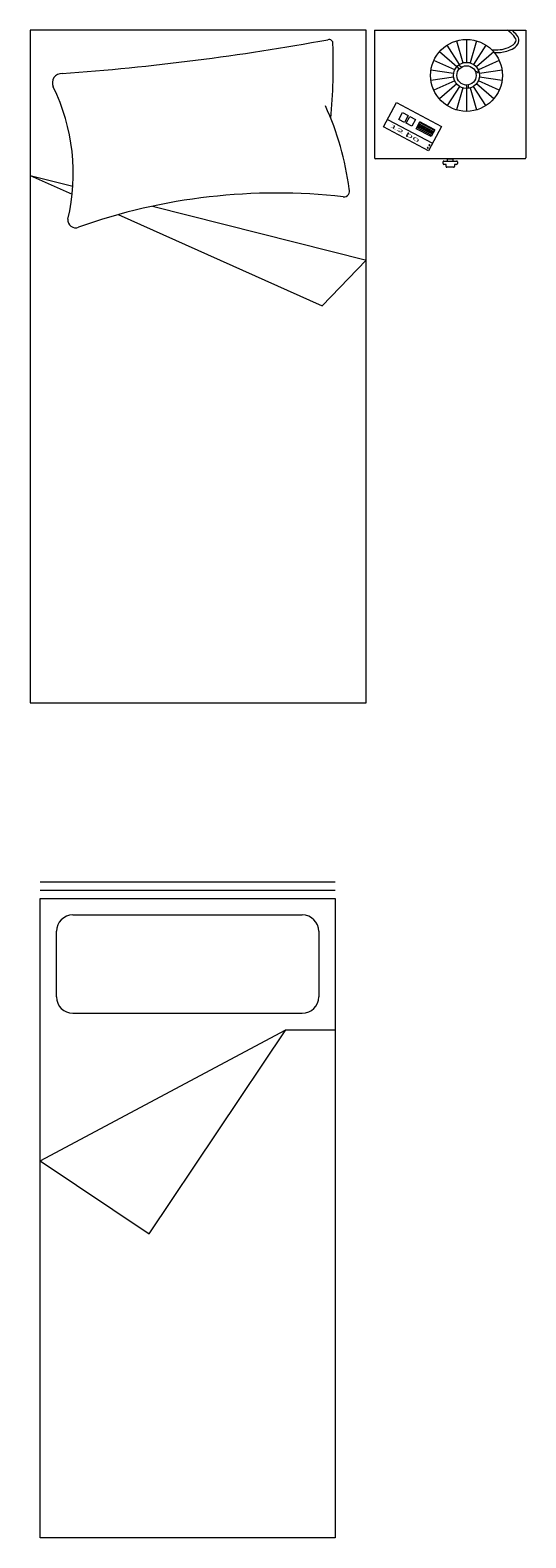
# Model space of a CAD drawing. Units: inches. Extents: x 1994 to 3075, y 3517 to 3950.
# Tile 2 of 58: x 1993.694 to 1993.7535, y 3553.3285 to 3553.5095. Entities that reach past the tile are written whole.
import ezdxf

# ---------------------------------------------------------------- set-up
doc = ezdxf.new("R2010")
doc.units = ezdxf.units.IN
doc.layers.add('A-FURN-REFR', color=8, linetype='Continuous', lineweight=13)
doc.layers.add('A-FURN-REFR-TEXT', color=7, linetype='Continuous', lineweight=13)
doc.styles.get("Standard").update_dxf_attribs({"font": 'arial.ttf'})

msp = doc.modelspace()

# ---------------------------------------------------------------- linework, layer by layer
at = {"layer": 'A-FURN-REFR'}
for p, q in [((1993.693973156495, 3553.509506909899), (1993.693973156495, 3553.428737082427)), ((1993.734358070231, 3553.509506909899), (1993.693973156495, 3553.509506909899)), ((1993.734358070231, 3553.509506909899), (1993.693973156495, 3553.509506909899)), ((1993.693973156495, 3553.509506909899), (1993.693973156495, 3553.428737082427)), ((1993.734358070231, 3553.494062278381), (1993.734358070231, 3553.509506909899)), ((1993.735351357589, 3553.509506909899), (1993.753524568771, 3553.509506909899)), ((1993.735351357589, 3553.509506909899), (1993.753524568771, 3553.509506909899)), ((1993.735351357589, 3553.509506909899), (1993.735351357589, 3553.494156783539)), ((1993.745181403067, 3553.508216216299), (1993.745956989547, 3553.505574811319)), ((1993.746397474044, 3553.50839106091), (1993.746397474044, 3553.505638143428)), ((1993.746397474044, 3553.50839106091), (1993.746397474044, 3553.505638143428)), ((1993.747613545022, 3553.508216216299), (1993.746837958541, 3553.505574811319)), ((1993.753524568771, 3553.509506909899), (1993.753524568771, 3553.494156783539)), ((1993.74521587127, 3553.505098523523), (1993.743135355055, 3553.506901301085)), ((1993.745552190485, 3553.505389945782), (1993.744063850928, 3553.507705847338)), ((1993.748731097161, 3553.507705847338), (1993.747242757603, 3553.505389945782)), ((1993.749659593034, 3553.506901301085), (1993.747579076819, 3553.505098523523)), ((1993.744849903524, 3553.504297165939), (1993.742125006773, 3553.504688946945)), ((1993.744975278483, 3553.504724153839), (1993.742471136662, 3553.505867757091)), ((1993.745502849012, 3553.504810658368), (1993.74527859826, 3553.505166721564)), ((1993.745785450507, 3553.505058262657), (1993.745427824392, 3553.505301143074)), ((1993.747449692653, 3553.504559308434), (1993.747859921791, 3553.5046275879)), ((1993.747528821771, 3553.504323860619), (1993.747904789476, 3553.504489970933)), ((1993.750323811427, 3553.505867757091), (1993.747819669605, 3553.504724153839)), ((1993.750669941316, 3553.504688946945), (1993.747945044565, 3553.504297165939)), ((1993.744849903524, 3553.50385215184), (1993.742125006773, 3553.503460370834)), ((1993.744975278483, 3553.503425163939), (1993.742471136662, 3553.502281560688)), ((1993.74521587127, 3553.503050794257), (1993.743135355055, 3553.501248016694)), ((1993.745552190485, 3553.502759371998), (1993.744063850928, 3553.50044347044)), ((1993.745956989547, 3553.50257450646), (1993.745181403067, 3553.49993310148)), ((1993.746339752154, 3553.502917629346), (1993.746441747398, 3553.502511801323)), ((1993.746608036915, 3553.502935487059), (1993.746605188935, 3553.502525033636)), ((1993.746837958541, 3553.50257450646), (1993.747613545022, 3553.49993310148)), ((1993.748731097161, 3553.50044347044), (1993.747242757603, 3553.502759371998)), ((1993.749659593034, 3553.501248016694), (1993.747579076819, 3553.503050794257)), ((1993.750323811427, 3553.502281560688), (1993.747819669605, 3553.503425163939)), ((1993.750669941316, 3553.503460370834), (1993.747945044565, 3553.50385215184)), ((1993.736434431094, 3553.497880184146), (1993.737989059791, 3553.500812799431)), ((1993.737989059791, 3553.500812799431), (1993.743398065434, 3553.497945394546)), ((1993.746397474044, 3553.50251117435), (1993.746397474044, 3553.499758256869)), ((1993.746397474044, 3553.50251117435), (1993.746397474044, 3553.499758256869)), ((1993.738265302491, 3553.498787983474), (1993.738702914558, 3553.499613484663)), ((1993.738702914558, 3553.499613484663), (1993.73938684813, 3553.49925091997)), ((1993.73938684813, 3553.49925091997), (1993.738949236063, 3553.498425418782)), ((1993.73914577831, 3553.49832122843), (1993.739583390378, 3553.499146729618)), ((1993.739583390378, 3553.499146729618), (1993.74026732395, 3553.498784164926)), ((1993.741843436736, 3553.495012779261), (1993.736434431094, 3553.497880184146)), ((1993.736919052996, 3553.498794363591), (1993.742328058639, 3553.495926958706)), ((1993.738949236063, 3553.498425418782), (1993.738265302491, 3553.498787983474)), ((1993.739829711883, 3553.497958663738), (1993.73914577831, 3553.49832122843)), ((1993.74026732395, 3553.498784164926), (1993.739829711883, 3553.497958663738)), ((1993.740361048673, 3553.497676993167), (1993.74079866074, 3553.498502494355)), ((1993.742146892584, 3553.496730287267), (1993.740361048673, 3553.497676993167)), ((1993.742223140979, 3553.496874120459), (1993.740437297068, 3553.497820826359)), ((1993.74229359681, 3553.497007026692), (1993.740507752898, 3553.497953732593)), ((1993.74233827728, 3553.497091310889), (1993.740552433369, 3553.498038016789)), ((1993.742390260616, 3553.497189371041), (1993.740604416705, 3553.498136076941)), ((1993.742449545936, 3553.497301205484), (1993.740663702025, 3553.498247911385)), ((1993.742532673235, 3553.497458014881), (1993.740746829324, 3553.498404720781)), ((1993.742584504651, 3553.497555788455), (1993.74079866074, 3553.498502494355)), ((1993.743398065434, 3553.497945394546), (1993.741843436736, 3553.495012779261)), ((1993.742584504651, 3553.497555788455), (1993.742146892584, 3553.496730287267)), ((1993.734358070231, 3553.428737082427), (1993.734358070231, 3553.494062278381)), ((1993.734358070231, 3553.428737082427), (1993.734358070231, 3553.494062278381)), ((1993.753430063613, 3553.494062278381), (1993.735445862748, 3553.494062278381)), ((1993.743576237704, 3553.493486644492), (1993.743576237704, 3553.493697253739)), ((1993.743670742862, 3553.493791758898), (1993.745205183498, 3553.493791758898)), ((1993.744119057778, 3553.493791758898), (1993.744119057778, 3553.494062278381)), ((1993.744119057778, 3553.494062278381), (1993.744756868582, 3553.494062278381)), ((1993.744756868582, 3553.494062278381), (1993.744756868582, 3553.493791758898)), ((1993.745299688657, 3553.493697253739), (1993.745299688657, 3553.493486644492)), ((1993.693973156495, 3553.492073330311), (1993.699103995308, 3553.490778399019)), ((1993.693973156495, 3553.492073330311), (1993.699023009254, 3553.489818449938)), ((1993.743932806685, 3553.493392139334), (1993.743670742862, 3553.493392139334)), ((1993.743932806685, 3553.493140378367), (1993.743932806685, 3553.493392139334)), ((1993.744848614517, 3553.493045873208), (1993.744027311843, 3553.493045873208)), ((1993.744943119676, 3553.493297634175), (1993.744943119676, 3553.493140378367)), ((1993.745205183498, 3553.493392139334), (1993.745037624834, 3553.493392139334)), ((1993.70866538292, 3553.488365277022), (1993.734368925486, 3553.481878165893)), ((1993.704544393294, 3553.487353019538), (1993.729037478722, 3553.476416269449)), ((1993.729037478722, 3553.476416269449), (1993.734358070231, 3553.481880905564)), ((1993.693973156495, 3553.428737082427), (1993.734358070231, 3553.428737082427)), ((1993.693973156495, 3553.428737082427), (1993.734358070231, 3553.428737082427)), ((1993.730607608411, 3553.407199015988), (1993.695174537545, 3553.407199015988)), ((1993.695174537545, 3553.40621476402), (1993.730607608411, 3553.40621476402)), ((1993.695174537545, 3553.405230512051), (1993.730607608411, 3553.405230512051)), ((1993.695174537545, 3553.328458858509), (1993.695174537545, 3553.405230512051)), ((1993.730607608411, 3553.405230512051), (1993.730607608411, 3553.328458858509)), ((1993.699111545419, 3553.403262008114), (1993.726670600537, 3553.403262008114)), ((1993.697143041482, 3553.393419488429), (1993.697143041482, 3553.401293504177)), ((1993.728639104475, 3553.401293504177), (1993.728639104475, 3553.393419488429)), ((1993.699111545419, 3553.391450984492), (1993.726670600537, 3553.391450984492)), ((1993.695174537545, 3553.373734449059), (1993.7247020966, 3553.389482480555)), ((1993.708252487577, 3553.364961324247), (1993.7247020966, 3553.389482480555)), ((1993.7247020966, 3553.389482480555), (1993.730607608411, 3553.389482480555)), ((1993.695174537545, 3553.373734449059), (1993.708252487577, 3553.364961324247)), ((1993.730607608411, 3553.328458858509), (1993.695174537545, 3553.328458858509))]:
    msp.add_line(p, q, dxfattribs=at)
for radius in [0.0043164020201009, 0.0015634845390022, 0.0011584684638608]:
    msp.add_circle((1993.746397474044, 3553.504074658889), radius, dxfattribs=at)
for centre, radius, start, end in [((1993.675942904223, 3553.803106406129), 0.2996159645214513, 274.1894661396486, 280.345956739574), ((1993.72990138795, 3553.507939375016), 0.0004482907065646, 350.157018905503, 109.5558986651033), ((1993.66145435768, 3553.505316682034), 0.0689357559366832, 354.6669486061241, 2.116631318036676), ((1993.697735165656, 3553.503196718279), 0.0010985341214448, 84.97952421387143, 205.9936625746376), ((1993.675380079956, 3553.492296475177), 0.0237724360313189, 346.680428679662, 25.99366257463764), ((1993.697352058582, 3553.485866639567), 0.0352435291682938, 7.457332088483644, 24.3977020455474), ((1993.739404522017, 3553.497078028364), 5.53897148363e-05, 90, 270), ((1993.739404522017, 3553.497078028364), 5.53897148363e-05, 270, 90), ((1993.739232407068, 3553.496798113319), 5.53897148363e-05, 90, 270), ((1993.739232407068, 3553.496798113319), 5.53897148363e-05, 270, 90), ((1993.741729739261, 3553.495360625428), 5.53897148363e-05, 90, 270), ((1993.741729739261, 3553.495360625428), 5.53897148363e-05, 270, 90), ((1993.741929866979, 3553.495710221951), 5.53897148363e-05, 90, 270), ((1993.741929866979, 3553.495710221951), 5.53897148363e-05, 270, 90), ((1993.735445862748, 3553.494156783539), 9.45051583805e-05, 180, 270), ((1993.743670742862, 3553.493697253739), 9.45051583805e-05, 90, 180), ((1993.743670742862, 3553.493486644492), 9.45051583805e-05, 180, 270), ((1993.745205183498, 3553.493697253739), 9.45051583805e-05, 0, 90), ((1993.745205183498, 3553.493486644492), 9.45051583805e-05, 270, 0), ((1993.753430063613, 3553.494156783539), 9.45051583805e-05, 270, 0), ((1993.744027311843, 3553.493140378367), 9.45051583805e-05, 180, 270), ((1993.744848614517, 3553.493140378367), 9.45051583805e-05, 270, 0), ((1993.745037624834, 3553.493297634175), 9.45051583805e-05, 90, 180), ((1993.723575036928, 3553.418772173519), 0.0711723108928985, 83.53797831642504, 109.5152363664946), ((1993.731662527122, 3553.490175932616), 0.0006880002040652, 263.537978316425, 22.64447096621987), ((1993.699414422063, 3553.486682357928), 0.0009117868872928, 171.3346578780885, 294.9744503598286), ((1993.699111545419, 3553.401293504177), 0.0019685039370079, 90, 180), ((1993.726670600537, 3553.401293504177), 0.0019685039370079, 0, 90), ((1993.699111545419, 3553.393419488429), 0.0019685039370079, 180, 270), ((1993.726670600537, 3553.393419488429), 0.0019685039370079, 270, 0)]:
    msp.add_arc(centre, radius, start, end, dxfattribs=at)
for points, knots in [([(1993.749434473615, 3553.507141898692), (1993.750087722963, 3553.507129666116), (1993.751110194962, 3553.507122829164), (1993.752837349823, 3553.50824735612), (1993.751893658769, 3553.509039273289), (1993.751328209425, 3553.509506909899)], [0, 0, 0, 0, 0.0020194675198324, 0.0031659294015444, 0.0048546887781589, 0.0048546887781589, 0.0048546887781589, 0.0048546887781589]), ([(1993.749735116114, 3553.506811714207), (1993.750207365685, 3553.506807864872), (1993.750708603079, 3553.506828132084), (1993.751775252321, 3553.507161301098), (1993.752447335162, 3553.507413028947), (1993.752809109176, 3553.50856758751), (1993.752409139887, 3553.508987861619), (1993.751963520491, 3553.509395740702), (1993.751899928874, 3553.509451597455), (1993.751835414037, 3553.509506909899)], [0.0077183477163671, 0.0077183477163671, 0.0077183477163671, 0.0077183477163671, 0.0428867239757183, 0.0428867239757183, 0.0785443346356031, 0.0785443346356031, 0.1084777623087474, 0.1084777623087474, 0.1132872864949097, 0.1132872864949097, 0.1132872864949097, 0.1132872864949097])]:
    msp.add_open_spline(points, degree=3, knots=knots, dxfattribs=at)

# ---------------------------------------------------------------- texts
at = {"layer": 'A-FURN-REFR-TEXT', "width": 3}
msp.add_text('12 00', height=0.000395772154613, rotation=330.6435157060532, dxfattribs=at).set_placement((1993.737161429086, 3553.497933836087))

doc.saveas('drawing.dxf')
